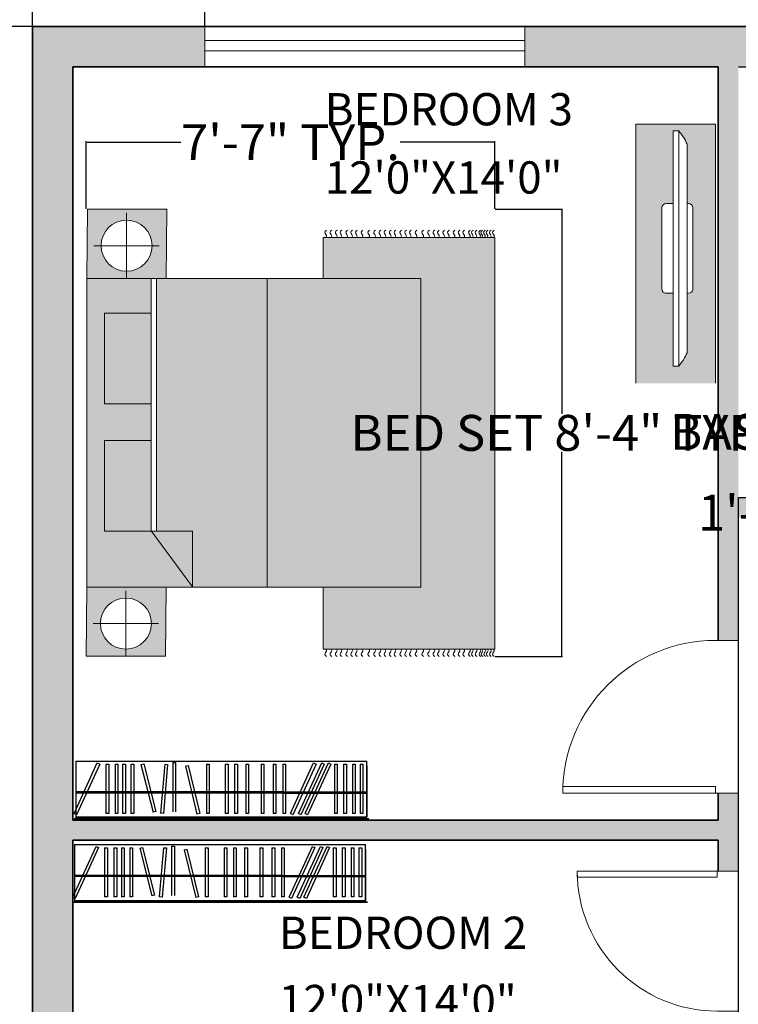
# Model space of a CAD drawing. Units: inches. Extents: x 853 to 1550, y 485 to 1596.
# Tile 13 of 18: x 979 to 1139, y 1208 to 1428. Entities that reach past the tile are written whole.
import ezdxf

# ---------------------------------------------------------------- set-up
doc = ezdxf.new("R2010")
doc.units = ezdxf.units.IN
doc.header["$MEASUREMENT"] = 0
for name, color, linetype, lineweight in [('A-ANNO-DIMS', 2, 'Continuous', 18), ('A-AREA-IDEN', 250, 'Continuous', 18), ('A-DOOR', 4, 'Continuous', 18), ('A-WALL-PATT', 250, 'Continuous', 13), ('closet', 32, 'Continuous', 25), ('furniture', 250, 'Continuous', 18), ('walls', 250, 'Continuous', 35), ('windows', 4, 'Continuous', 18)]:
    doc.layers.add(name, color=color, linetype=linetype, lineweight=lineweight)
doc.layers.add('A-FURN-PATT', color=254, linetype='Continuous', lineweight=13, true_color=0xfeeab9)
doc.styles.get("Standard").update_dxf_attribs({"font": 'arial.ttf'})
doc.dimstyles.get("Standard").update_dxf_attribs({"dimtxt": 8, "dimasz": 0.18, "dimexe": 0.18, "dimexo": 0.0625, "dimgap": 0.09, "dimtad": 0, "dimtih": 1, "dimtoh": 1, "dimzin": 0, "dimdsep": 46, "dimlunit": 3, "dimtxsty": 'Standard', "dimcen": 0.09, "dimadec": 0, "dimazin": 0, "dimtfac": 1, "dimtofl": 0, "dimtmove": 0, "dimatfit": 3, "dimfxl": 1, "dimtolj": 1, "dimtzin": 0, "dimarcsym": 0})

# ---------------------------------------------------------------- blocks, each defined once
blk = doc.blocks.new('CARPET')
at = {"layer": 'furniture'}
for p, q in [((-51.53, -98.11), (-51.53, -55.12)), ((-51.53, -55.12), (-41.27, -55.12)), ((36, -55.12), (51.55, -55.12)), ((51.55, -55.12), (51.55, -98.11)), ((51.55, -98.11), (-51.53, -98.11))]:
    blk.add_line(p, q, dxfattribs=at)
for points, knots in [([(-53.37, -55.99), (-53.22, -55.8), (-52.9, -55.41), (-52.34, -55.8), (-51.89, -56.08), (-51.65, -55.91), (-51.53, -55.83)], [0, 0, 0, 0, 0.653278, 1.290138, 1.740457, 2.114451, 2.114451, 2.114451, 2.114451]), ([(53.37, -55.99), (53.22, -55.8), (52.9, -55.41), (52.34, -55.8), (51.89, -56.08), (51.65, -55.91), (51.53, -55.83)], [0, 0, 0, 0, 0.653278, 1.290138, 1.740457, 2.114451, 2.114451, 2.114451, 2.114451]), ([(-53.37, -57.26), (-53.22, -57.07), (-52.9, -56.67), (-52.34, -57.07), (-51.89, -57.35), (-51.65, -57.17), (-51.53, -57.1)], [0, 0, 0, 0, 0.653278, 1.290138, 1.740457, 2.114451, 2.114451, 2.114451, 2.114451]), ([(-53.37, -58.59), (-53.22, -58.4), (-52.9, -58.01), (-52.34, -58.4), (-51.89, -58.68), (-51.65, -58.5), (-51.53, -58.43)], [0, 0, 0, 0, 0.653278, 1.290138, 1.740457, 2.114451, 2.114451, 2.114451, 2.114451]), ([(53.37, -57.26), (53.22, -57.07), (52.9, -56.67), (52.34, -57.07), (51.89, -57.35), (51.65, -57.17), (51.53, -57.1)], [0, 0, 0, 0, 0.653278, 1.290138, 1.740457, 2.114451, 2.114451, 2.114451, 2.114451]), ([(53.37, -58.59), (53.22, -58.4), (52.9, -58.01), (52.34, -58.4), (51.89, -58.68), (51.65, -58.5), (51.53, -58.43)], [0, 0, 0, 0, 0.653278, 1.290138, 1.740457, 2.114451, 2.114451, 2.114451, 2.114451]), ([(-53.37, -59.78), (-53.22, -59.58), (-52.9, -59.19), (-52.34, -59.58), (-51.89, -59.86), (-51.65, -59.69), (-51.53, -59.61)], [0, 0, 0, 0, 0.653278, 1.290138, 1.740457, 2.114451, 2.114451, 2.114451, 2.114451]), ([(-53.37, -61.22), (-53.22, -61.02), (-52.9, -60.63), (-52.34, -61.02), (-51.89, -61.3), (-51.65, -61.13), (-51.53, -61.05)], [0, 0, 0, 0, 0.653278, 1.290138, 1.740457, 2.114451, 2.114451, 2.114451, 2.114451]), ([(53.37, -59.78), (53.22, -59.58), (52.9, -59.19), (52.34, -59.58), (51.89, -59.86), (51.65, -59.69), (51.53, -59.61)], [0, 0, 0, 0, 0.653278, 1.290138, 1.740457, 2.114451, 2.114451, 2.114451, 2.114451]), ([(53.37, -61.22), (53.22, -61.02), (52.9, -60.63), (52.34, -61.02), (51.89, -61.3), (51.65, -61.13), (51.53, -61.05)], [0, 0, 0, 0, 0.653278, 1.290138, 1.740457, 2.114451, 2.114451, 2.114451, 2.114451]), ([(-53.37, -62.44), (-53.22, -62.25), (-52.9, -61.86), (-52.34, -62.25), (-51.89, -62.53), (-51.65, -62.36), (-51.53, -62.28)], [0, 0, 0, 0, 0.653278, 1.290138, 1.740457, 2.114451, 2.114451, 2.114451, 2.114451]), ([(-53.37, -63.63), (-53.22, -63.43), (-52.9, -63.04), (-52.34, -63.43), (-51.89, -63.72), (-51.65, -63.54), (-51.53, -63.46)], [0, 0, 0, 0, 0.653278, 1.290138, 1.740457, 2.114451, 2.114451, 2.114451, 2.114451]), ([(53.37, -62.44), (53.22, -62.25), (52.9, -61.86), (52.34, -62.25), (51.89, -62.53), (51.65, -62.36), (51.53, -62.28)], [0, 0, 0, 0, 0.653278, 1.290138, 1.740457, 2.114451, 2.114451, 2.114451, 2.114451]), ([(53.37, -63.63), (53.22, -63.43), (52.9, -63.04), (52.34, -63.43), (51.89, -63.72), (51.65, -63.54), (51.53, -63.46)], [0, 0, 0, 0, 0.653278, 1.290138, 1.740457, 2.114451, 2.114451, 2.114451, 2.114451]), ([(-53.37, -65.07), (-53.22, -64.87), (-52.9, -64.48), (-52.34, -64.87), (-51.89, -65.15), (-51.65, -64.98), (-51.53, -64.9)], [0, 0, 0, 0, 0.653278, 1.290138, 1.740457, 2.114451, 2.114451, 2.114451, 2.114451]), ([(-53.37, -66.76), (-53.22, -66.56), (-52.9, -66.17), (-52.34, -66.56), (-51.89, -66.84), (-51.65, -66.67), (-51.53, -66.59)], [0, 0, 0, 0, 0.653278, 1.290138, 1.740457, 2.114451, 2.114451, 2.114451, 2.114451]), ([(53.37, -65.07), (53.22, -64.87), (52.9, -64.48), (52.34, -64.87), (51.89, -65.15), (51.65, -64.98), (51.53, -64.9)], [0, 0, 0, 0, 0.653278, 1.290138, 1.740457, 2.114451, 2.114451, 2.114451, 2.114451]), ([(53.37, -66.76), (53.22, -66.56), (52.9, -66.17), (52.34, -66.56), (51.89, -66.84), (51.65, -66.67), (51.53, -66.59)], [0, 0, 0, 0, 0.653278, 1.290138, 1.740457, 2.114451, 2.114451, 2.114451, 2.114451]), ([(-53.37, -68.2), (-53.22, -68), (-52.9, -67.61), (-52.34, -68), (-51.89, -68.28), (-51.65, -68.11), (-51.53, -68.03)], [0, 0, 0, 0, 0.653278, 1.290138, 1.740457, 2.114451, 2.114451, 2.114451, 2.114451]), ([(53.37, -68.2), (53.22, -68), (52.9, -67.61), (52.34, -68), (51.89, -68.28), (51.65, -68.11), (51.53, -68.03)], [0, 0, 0, 0, 0.653278, 1.290138, 1.740457, 2.114451, 2.114451, 2.114451, 2.114451]), ([(-53.37, -69.53), (-53.22, -69.33), (-52.9, -68.94), (-52.34, -69.33), (-51.89, -69.61), (-51.65, -69.44), (-51.53, -69.36)], [0, 0, 0, 0, 0.653278, 1.290138, 1.740457, 2.114451, 2.114451, 2.114451, 2.114451]), ([(-53.37, -70.79), (-53.22, -70.6), (-52.9, -70.21), (-52.34, -70.6), (-51.89, -70.88), (-51.65, -70.7), (-51.53, -70.63)], [0, 0, 0, 0, 0.653278, 1.290138, 1.740457, 2.114451, 2.114451, 2.114451, 2.114451]), ([(53.37, -69.53), (53.22, -69.33), (52.9, -68.94), (52.34, -69.33), (51.89, -69.61), (51.65, -69.44), (51.53, -69.36)], [0, 0, 0, 0, 0.653278, 1.290138, 1.740457, 2.114451, 2.114451, 2.114451, 2.114451]), ([(53.37, -70.79), (53.22, -70.6), (52.9, -70.21), (52.34, -70.6), (51.89, -70.88), (51.65, -70.7), (51.53, -70.63)], [0, 0, 0, 0, 0.653278, 1.290138, 1.740457, 2.114451, 2.114451, 2.114451, 2.114451]), ([(-53.37, -72.12), (-53.22, -71.93), (-52.9, -71.54), (-52.34, -71.93), (-51.89, -72.21), (-51.65, -72.04), (-51.53, -71.96)], [0, 0, 0, 0, 0.653278, 1.290138, 1.740457, 2.114451, 2.114451, 2.114451, 2.114451]), ([(-53.37, -73.31), (-53.22, -73.11), (-52.9, -72.72), (-52.34, -73.11), (-51.89, -73.4), (-51.65, -73.22), (-51.53, -73.14)], [0, 0, 0, 0, 0.653278, 1.290138, 1.740457, 2.114451, 2.114451, 2.114451, 2.114451]), ([(53.37, -72.12), (53.22, -71.93), (52.9, -71.54), (52.34, -71.93), (51.89, -72.21), (51.65, -72.04), (51.53, -71.96)], [0, 0, 0, 0, 0.653278, 1.290138, 1.740457, 2.114451, 2.114451, 2.114451, 2.114451]), ([(53.37, -73.31), (53.22, -73.11), (52.9, -72.72), (52.34, -73.11), (51.89, -73.4), (51.65, -73.22), (51.53, -73.14)], [0, 0, 0, 0, 0.653278, 1.290138, 1.740457, 2.114451, 2.114451, 2.114451, 2.114451]), ([(-53.37, -74.75), (-53.22, -74.55), (-52.9, -74.16), (-52.34, -74.55), (-51.89, -74.83), (-51.65, -74.66), (-51.53, -74.58)], [0, 0, 0, 0, 0.653278, 1.290138, 1.740457, 2.114451, 2.114451, 2.114451, 2.114451]), ([(-53.37, -75.98), (-53.22, -75.78), (-52.9, -75.39), (-52.34, -75.78), (-51.89, -76.06), (-51.65, -75.89), (-51.53, -75.81)], [0, 0, 0, 0, 0.653278, 1.290138, 1.740457, 2.114451, 2.114451, 2.114451, 2.114451]), ([(53.37, -74.75), (53.22, -74.55), (52.9, -74.16), (52.34, -74.55), (51.89, -74.83), (51.65, -74.66), (51.53, -74.58)], [0, 0, 0, 0, 0.653278, 1.290138, 1.740457, 2.114451, 2.114451, 2.114451, 2.114451]), ([(53.37, -75.98), (53.22, -75.78), (52.9, -75.39), (52.34, -75.78), (51.89, -76.06), (51.65, -75.89), (51.53, -75.81)], [0, 0, 0, 0, 0.653278, 1.290138, 1.740457, 2.114451, 2.114451, 2.114451, 2.114451]), ([(-53.37, -77.16), (-53.22, -76.96), (-52.9, -76.57), (-52.34, -76.96), (-51.89, -77.25), (-51.65, -77.07), (-51.53, -76.99)], [0, 0, 0, 0, 0.653278, 1.290138, 1.740457, 2.114451, 2.114451, 2.114451, 2.114451]), ([(-53.37, -78.6), (-53.22, -78.4), (-52.9, -78.01), (-52.34, -78.4), (-51.89, -78.68), (-51.65, -78.51), (-51.53, -78.43)], [0, 0, 0, 0, 0.653278, 1.290138, 1.740457, 2.114451, 2.114451, 2.114451, 2.114451]), ([(53.37, -77.16), (53.22, -76.96), (52.9, -76.57), (52.34, -76.96), (51.89, -77.25), (51.65, -77.07), (51.53, -76.99)], [0, 0, 0, 0, 0.653278, 1.290138, 1.740457, 2.114451, 2.114451, 2.114451, 2.114451]), ([(53.37, -78.6), (53.22, -78.4), (52.9, -78.01), (52.34, -78.4), (51.89, -78.68), (51.65, -78.51), (51.53, -78.43)], [0, 0, 0, 0, 0.653278, 1.290138, 1.740457, 2.114451, 2.114451, 2.114451, 2.114451]), ([(-53.37, -80.29), (-53.22, -80.09), (-52.9, -79.7), (-52.34, -80.09), (-51.89, -80.37), (-51.65, -80.2), (-51.53, -80.12)], [0, 0, 0, 0, 0.653278, 1.290138, 1.740457, 2.114451, 2.114451, 2.114451, 2.114451]), ([(-53.37, -81.73), (-53.22, -81.53), (-52.9, -81.14), (-52.34, -81.53), (-51.89, -81.81), (-51.65, -81.64), (-51.53, -81.56)], [0, 0, 0, 0, 0.653278, 1.290138, 1.740457, 2.114451, 2.114451, 2.114451, 2.114451]), ([(53.37, -80.29), (53.22, -80.09), (52.9, -79.7), (52.34, -80.09), (51.89, -80.37), (51.65, -80.2), (51.53, -80.12)], [0, 0, 0, 0, 0.653278, 1.290138, 1.740457, 2.114451, 2.114451, 2.114451, 2.114451]), ([(53.37, -81.73), (53.22, -81.53), (52.9, -81.14), (52.34, -81.53), (51.89, -81.81), (51.65, -81.64), (51.53, -81.56)], [0, 0, 0, 0, 0.653278, 1.290138, 1.740457, 2.114451, 2.114451, 2.114451, 2.114451]), ([(-53.37, -83.06), (-53.22, -82.86), (-52.9, -82.47), (-52.34, -82.86), (-51.89, -83.14), (-51.65, -82.97), (-51.53, -82.89)], [0, 0, 0, 0, 0.653278, 1.290138, 1.740457, 2.114451, 2.114451, 2.114451, 2.114451]), ([(-53.37, -84.18), (-53.22, -83.99), (-52.9, -83.6), (-52.34, -83.99), (-51.89, -84.27), (-51.65, -84.09), (-51.53, -84.02)], [0, 0, 0, 0, 0.653278, 1.290138, 1.740457, 2.114451, 2.114451, 2.114451, 2.114451]), ([(53.37, -83.06), (53.22, -82.86), (52.9, -82.47), (52.34, -82.86), (51.89, -83.14), (51.65, -82.97), (51.53, -82.89)], [0, 0, 0, 0, 0.653278, 1.290138, 1.740457, 2.114451, 2.114451, 2.114451, 2.114451]), ([(53.37, -84.18), (53.22, -83.99), (52.9, -83.6), (52.34, -83.99), (51.89, -84.27), (51.65, -84.09), (51.53, -84.02)], [0, 0, 0, 0, 0.653278, 1.290138, 1.740457, 2.114451, 2.114451, 2.114451, 2.114451]), ([(-53.37, -85.51), (-53.22, -85.32), (-52.9, -84.93), (-52.34, -85.32), (-51.89, -85.6), (-51.65, -85.42), (-51.53, -85.35)], [0, 0, 0, 0, 0.653278, 1.290138, 1.740457, 2.114451, 2.114451, 2.114451, 2.114451]), ([(-53.37, -86.7), (-53.22, -86.5), (-52.9, -86.11), (-52.34, -86.5), (-51.89, -86.78), (-51.65, -86.61), (-51.53, -86.53)], [0, 0, 0, 0, 0.653278, 1.290138, 1.740457, 2.114451, 2.114451, 2.114451, 2.114451]), ([(53.37, -85.51), (53.22, -85.32), (52.9, -84.93), (52.34, -85.32), (51.89, -85.6), (51.65, -85.42), (51.53, -85.35)], [0, 0, 0, 0, 0.653278, 1.290138, 1.740457, 2.114451, 2.114451, 2.114451, 2.114451]), ([(53.37, -86.7), (53.22, -86.5), (52.9, -86.11), (52.34, -86.5), (51.89, -86.78), (51.65, -86.61), (51.53, -86.53)], [0, 0, 0, 0, 0.653278, 1.290138, 1.740457, 2.114451, 2.114451, 2.114451, 2.114451]), ([(-53.37, -88.14), (-53.22, -87.94), (-52.9, -87.55), (-52.34, -87.94), (-51.89, -88.22), (-51.65, -88.05), (-51.53, -87.97)], [0, 0, 0, 0, 0.653278, 1.290138, 1.740457, 2.114451, 2.114451, 2.114451, 2.114451]), ([(53.37, -88.14), (53.22, -87.94), (52.9, -87.55), (52.34, -87.94), (51.89, -88.22), (51.65, -88.05), (51.53, -87.97)], [0, 0, 0, 0, 0.653278, 1.290138, 1.740457, 2.114451, 2.114451, 2.114451, 2.114451]), ([(-53.37, -89.36), (-53.22, -89.17), (-52.9, -88.78), (-52.34, -89.17), (-51.89, -89.45), (-51.65, -89.28), (-51.53, -89.2)], [0, 0, 0, 0, 0.653278, 1.290138, 1.740457, 2.114451, 2.114451, 2.114451, 2.114451]), ([(-53.37, -90.55), (-53.22, -90.35), (-52.9, -89.96), (-52.34, -90.35), (-51.89, -90.64), (-51.65, -90.46), (-51.53, -90.38)], [0, 0, 0, 0, 0.653278, 1.290138, 1.740457, 2.114451, 2.114451, 2.114451, 2.114451]), ([(53.37, -89.36), (53.22, -89.17), (52.9, -88.78), (52.34, -89.17), (51.89, -89.45), (51.65, -89.28), (51.53, -89.2)], [0, 0, 0, 0, 0.653278, 1.290138, 1.740457, 2.114451, 2.114451, 2.114451, 2.114451]), ([(53.37, -90.55), (53.22, -90.35), (52.9, -89.96), (52.34, -90.35), (51.9, -90.63), (51.66, -90.47), (51.55, -90.4)], [0, 0, 0, 0, 0.653278, 1.290138, 1.740457, 2.0926, 2.0926, 2.0926, 2.0926]), ([(-53.37, -91.99), (-53.22, -91.79), (-52.9, -91.4), (-52.34, -91.79), (-51.89, -92.07), (-51.65, -91.9), (-51.53, -91.82)], [0, 0, 0, 0, 0.653278, 1.290138, 1.740457, 2.114451, 2.114451, 2.114451, 2.114451]), ([(-53.37, -92.69), (-53.22, -92.48), (-52.9, -92.08), (-52.35, -92.49), (-51.89, -92.77), (-51.65, -92.6), (-51.53, -92.52)], [0, 0, 0, 0, 0.663904, 1.307406, 1.757725, 2.131719, 2.131719, 2.131719, 2.131719]), ([(-53.37, -93.61), (-53.22, -93.42), (-52.9, -93.03), (-52.34, -93.42), (-51.89, -93.7), (-51.65, -93.52), (-51.53, -93.45)], [0, 0, 0, 0, 0.653278, 1.290138, 1.740457, 2.114451, 2.114451, 2.114451, 2.114451]), ([(53.37, -91.99), (53.22, -91.79), (52.9, -91.4), (52.34, -91.79), (51.9, -92.07), (51.66, -91.91), (51.55, -91.83)], [0, 0, 0, 0, 0.653278, 1.290138, 1.740457, 2.0926, 2.0926, 2.0926, 2.0926]), ([(53.37, -92.69), (53.22, -92.49), (52.9, -92.09), (52.34, -92.49), (51.9, -92.77), (51.66, -92.61), (51.55, -92.53)], [0, 0, 0, 0, 0.656792, 1.295826, 1.746145, 2.098292, 2.098292, 2.098292, 2.098292]), ([(53.37, -93.66), (53.22, -93.46), (52.9, -93.07), (52.34, -93.46), (51.9, -93.74), (51.66, -93.58), (51.55, -93.5)], [0, 0, 0, 0, 0.653278, 1.290138, 1.740457, 2.0926, 2.0926, 2.0926, 2.0926]), ([(-53.37, -94.55), (-53.22, -94.35), (-52.9, -93.96), (-52.34, -94.35), (-51.89, -94.63), (-51.65, -94.46), (-51.53, -94.38)], [0, 0, 0, 0, 0.653278, 1.290138, 1.740457, 2.114451, 2.114451, 2.114451, 2.114451]), ([(-53.37, -95.05), (-53.22, -94.85), (-52.9, -94.46), (-52.34, -94.85), (-51.89, -95.14), (-51.65, -94.96), (-51.53, -94.88)], [0, 0, 0, 0, 0.653278, 1.290138, 1.740457, 2.114451, 2.114451, 2.114451, 2.114451]), ([(-53.37, -95.73), (-53.22, -95.54), (-52.9, -95.15), (-52.34, -95.54), (-51.89, -95.82), (-51.65, -95.65), (-51.53, -95.57)], [0, 0, 0, 0, 0.653278, 1.290138, 1.740457, 2.114451, 2.114451, 2.114451, 2.114451]), ([(-53.37, -96.38), (-53.22, -96.18), (-52.9, -95.79), (-52.34, -96.18), (-51.89, -96.47), (-51.65, -96.29), (-51.53, -96.21)], [0, 0, 0, 0, 0.653278, 1.290138, 1.740457, 2.114451, 2.114451, 2.114451, 2.114451]), ([(53.37, -95.78), (53.22, -95.58), (52.9, -95.19), (52.34, -95.58), (51.89, -95.86), (51.65, -95.69), (51.53, -95.61)], [0, 0, 0, 0, 0.653278, 1.290138, 1.740457, 2.114451, 2.114451, 2.114451, 2.114451]), ([(53.37, -96.43), (53.22, -96.23), (52.9, -95.84), (52.34, -96.23), (51.89, -96.51), (51.65, -96.34), (51.53, -96.26)], [0, 0, 0, 0, 0.653278, 1.290138, 1.740457, 2.114451, 2.114451, 2.114451, 2.114451]), ([(53.37, -94.59), (53.22, -94.4), (52.9, -94.01), (52.34, -94.4), (51.9, -94.68), (51.66, -94.51), (51.55, -94.44)], [0, 0, 0, 0, 0.653278, 1.290138, 1.740457, 2.0926, 2.0926, 2.0926, 2.0926]), ([(53.37, -95.1), (53.22, -94.9), (52.9, -94.51), (52.34, -94.9), (51.9, -95.18), (51.66, -95.02), (51.55, -94.94)], [0, 0, 0, 0, 0.653278, 1.290138, 1.740457, 2.0926, 2.0926, 2.0926, 2.0926]), ([(-53.37, -97.17), (-53.22, -96.98), (-52.9, -96.59), (-52.34, -96.98), (-51.89, -97.26), (-51.65, -97.08), (-51.53, -97.01)], [0, 0, 0, 0, 0.653278, 1.290138, 1.740457, 2.114451, 2.114451, 2.114451, 2.114451]), ([(-53.37, -97.99), (-53.22, -97.79), (-52.9, -97.4), (-52.34, -97.79), (-51.89, -98.08), (-51.65, -97.9), (-51.53, -97.82)], [0, 0, 0, 0, 0.653278, 1.290138, 1.740457, 2.114451, 2.114451, 2.114451, 2.114451]), ([(53.37, -97.22), (53.22, -97.02), (52.9, -96.63), (52.34, -97.02), (51.89, -97.3), (51.65, -97.13), (51.53, -97.05)], [0, 0, 0, 0, 0.653278, 1.290138, 1.740457, 2.114451, 2.114451, 2.114451, 2.114451]), ([(53.37, -97.99), (53.22, -97.79), (52.9, -97.4), (52.34, -97.79), (51.89, -98.08), (51.65, -97.9), (51.53, -97.82)], [0, 0, 0, 0, 0.653278, 1.290138, 1.740457, 2.114451, 2.114451, 2.114451, 2.114451])]:
    blk.add_open_spline(points, degree=3, knots=knots, dxfattribs=at)
blk = doc.blocks.new('A$C58D270C6')
at = {"layer": 'furniture'}
for p, q in [((9.09, 124.13), (9.09, 108.87)), ((1.46, 116.5), (16.73, 116.5)), ((42.08, 108), (42.08, 36)), ((14.97, 94.84), (24.62, 107.92)), ((24.62, 94.93), (24.62, 107.92)), ((14.97, 94.93), (24.62, 94.93)), ((14.97, 94.84), (14.97, 36)), ((16.22, 94.93), (16.22, 36)), ((9.25, 36), (9.25, 20.74)), ((1.62, 28.37), (16.88, 28.37))]:
    blk.add_line(p, q, dxfattribs=at)
for points in [[(18.5, 108), (18.34, 124.13), (-0.16, 124.13), (0, 108)], [(0, 108), (77.91, 108), (77.91, 36), (0, 36)], [(4.09, 94.93), (14.97, 94.93), (14.97, 73.83), (4.09, 73.83)], [(4.09, 65.23), (14.97, 65.23), (14.97, 44.13), (4.09, 44.13)], [(18.65, 19.87), (18.5, 36), (0, 36), (0.16, 19.87)]]:
    blk.add_lwpolyline(points, close=True, dxfattribs=at)
for centre in [(9.09, 116.5), (9.25, 28.37)]:
    blk.add_circle(centre, 5.95, dxfattribs=at)
at = {"layer": 'furniture', "xscale": 0.9312884925094044, "yscale": 0.9312884925094044, "zscale": 0.9312884925094044, "rotation": 90}
blk.add_blockref('CARPET', (3.79, 74.47), dxfattribs=at)
blk = doc.blocks.new('*U10')
for p, q in [((0, 0), (0, -6)), ((40, 0), (40, -6))]:
    blk.add_line(p, q)
blk.add_lwpolyline([(0, 0), (0, 40), (1.75, 40), (1.75, 0)], close=True)
blk.add_arc((0, 0), 40, 0, 90)
blk = doc.blocks.new('WIN-71IN')
for p, q in [((0, 9), (0, 0)), ((71.43, 9), (0, 9)), ((0, 9), (0, 5.92)), ((71.43, 0), (71.43, 9)), ((0, 5.92), (71.43, 5.92)), ((71.43, 5.92), (71.43, 3.59)), ((71.43, 3.59), (0, 3.59)), ((0, 0), (71.43, 0))]:
    blk.add_line(p, q)
blk = doc.blocks.new('closet')
at = {"layer": 'closet'}
for p, q in [((-0.71, -5.58), (5.59, 8.19)), ((5.59, 8.19), (6.27, 7.88)), ((26.09, 8.25), (26.09, -5.1)), ((26.84, 8.25), (26.84, -5.1)), ((57.99, -5.58), (64.3, 8.19)), ((60.19, -5.58), (66.49, 8.19)), ((62, -5.58), (68.3, 8.19)), ((-0.23, 7.39), (-0.23, -6.57)), ((6.27, 7.88), (-0.04, -5.89)), ((7.92, 7.84), (8.68, 7.84)), ((7.92, 7.84), (7.92, -5.51)), ((8.68, 7.84), (8.68, -5.51)), ((10.44, 7.84), (11.2, 7.84)), ((10.44, 7.84), (10.44, -5.51)), ((11.2, 7.84), (11.2, -5.51)), ((12.45, 7.84), (13.21, 7.84)), ((12.45, 7.84), (12.45, -5.51)), ((13.21, 7.84), (13.21, -5.51)), ((14.71, 7.84), (15.47, 7.84)), ((14.71, 7.84), (14.71, -5.51)), ((15.47, 7.84), (15.47, -5.51)), ((17.44, 7.75), (18.17, 7.93)), ((17.44, 7.75), (20.73, -5.2)), ((18.17, 7.93), (21.46, -5.01)), ((23.92, 7.84), (22.75, -5.46)), ((24.67, 7.78), (23.51, -5.53)), ((23.92, 7.84), (24.67, 7.78)), ((29.49, 7.29), (32.64, -5.69)), ((30.22, 7.46), (33.37, -5.51)), ((35.23, 7.84), (35.23, -5.51)), ((35.99, 7.84), (35.99, -5.51)), ((40.33, 7.84), (40.33, -5.51)), ((41.08, 7.84), (41.08, -5.51)), ((42.85, 7.84), (42.85, -5.51)), ((43.61, 7.84), (43.61, -5.51)), ((45.9, 7.84), (45.9, -5.51)), ((46.65, 7.84), (46.65, -5.51)), ((50.07, 7.84), (50.07, -5.51)), ((50.82, 7.84), (50.82, -5.51)), ((53.32, 7.84), (53.32, -5.51)), ((54.08, 7.84), (54.08, -5.51)), ((55.9, 7.84), (55.9, -5.51)), ((56.65, 7.84), (56.65, -5.51)), ((64.97, 7.88), (58.67, -5.89)), ((67.17, 7.88), (60.87, -5.89)), ((68.98, 7.88), (62.67, -5.89)), ((69.96, 7.84), (69.96, -5.51)), ((70.72, 7.84), (70.72, -5.51)), ((72.43, 7.84), (72.43, -5.51)), ((73.19, 7.84), (73.19, -5.51)), ((74.82, 7.84), (74.82, -5.51)), ((75.57, 7.84), (75.57, -5.51)), ((76.94, 7.84), (76.94, -5.51)), ((77.69, 7.84), (77.69, -5.51)), ((56.23, 0.33), (0, 0.33)), ((56.2, 0), (0, 0)), ((56.2, 0), (78.76, 0)), ((56.23, 0.33), (78.76, 0.33)), ((21.46, -5.01), (20.73, -5.2)), ((-0.04, -5.89), (-0.71, -5.58)), ((23.51, -5.53), (22.75, -5.46)), ((33.37, -5.51), (32.64, -5.69)), ((35.99, -5.51), (35.23, -5.51)), ((41.08, -5.51), (40.33, -5.51)), ((43.61, -5.51), (42.85, -5.51)), ((46.65, -5.51), (45.9, -5.51)), ((50.82, -5.51), (50.07, -5.51)), ((54.08, -5.51), (53.32, -5.51)), ((56.65, -5.51), (55.9, -5.51)), ((58.67, -5.89), (57.99, -5.58)), ((60.87, -5.89), (60.19, -5.58)), ((62.67, -5.89), (62, -5.58)), ((70.72, -5.51), (69.96, -5.51)), ((73.19, -5.51), (72.43, -5.51)), ((75.57, -5.51), (74.82, -5.51)), ((77.69, -5.51), (76.94, -5.51))]:
    blk.add_line(p, q, dxfattribs=at)
blk = doc.blocks.new('rotated closet')
at = {"layer": 'closet'}
for p, q in [((26.32, 0.86), (27.07, 0.86)), ((29.72, -0.11), (30.45, 0.07)), ((35.46, 0.45), (36.22, 0.45)), ((40.56, 0.45), (41.31, 0.45)), ((43.08, 0.45), (43.84, 0.45)), ((46.13, 0.45), (46.88, 0.45)), ((50.3, 0.45), (51.05, 0.45)), ((53.56, 0.45), (54.31, 0.45)), ((56.13, 0.45), (56.88, 0.45)), ((64.53, 0.8), (65.2, 0.49)), ((66.72, 0.8), (67.4, 0.49)), ((68.53, 0.8), (69.21, 0.49)), ((70.19, 0.45), (70.95, 0.45)), ((72.66, 0.45), (73.42, 0.45)), ((75.05, 0.45), (75.81, 0.45)), ((77.17, 0.45), (77.92, 0.45)), ((78.99, 0), (78.99, -13.96)), ((8.91, -12.91), (8.15, -12.91)), ((11.43, -12.91), (10.67, -12.91)), ((13.44, -12.91), (12.68, -12.91)), ((15.7, -12.91), (14.94, -12.91)), ((-0.46, -14.27), (79.54, -14.27)), ((0, -13.96), (78.99, -13.96))]:
    blk.add_line(p, q, dxfattribs=at)
blk.add_blockref('closet', (0.23, -7.39), dxfattribs=at)
blk = doc.blocks.new('WARDROBE-FRAMED')
for p, q in [((0.4, 12.8), (65.33, 12.8)), ((0.4, 12.8), (0.4, 0.26)), ((65.33, 0.26), (65.33, 12.8)), ((0.02, 0), (65.79, 0)), ((65.33, 0.26), (0.4, 0.26)), ((0.4, 0.26), (0.4, 0))]:
    blk.add_line(p, q)
at = {"xscale": 0.8221057635095903, "yscale": 0.8221057635095903, "zscale": 0.8221057635095903, "rotation": 359.9999999992008}
blk.add_blockref('rotated closet', (0.4, 11.74), dxfattribs=at)
blk = doc.blocks.new('PLASMA-LARGE')
at = {"layer": 'furniture'}
for p, q in [((-7.26, 0), (7.26, 0)), ((-18.61, -1), (18.61, -1)), ((-8, -1), (-8, -0.74)), ((8, -1), (8, -0.74)), ((-21, -2.5), (21, -2.5)), ((-21, -2.5), (-21, -3.5)), ((-21, -3.5), (21, -3.5)), ((-8, -3.5), (-8, -4.76)), ((8, -3.5), (8, -4.76)), ((21, -2.5), (21, -3.5)), ((-7.26, -5.5), (7.26, -5.5))]:
    blk.add_line(p, q, dxfattribs=at)
for centre, radius, start, end in [((-7.26, -0.74), 0.744, 90, 180), ((7.26, -0.74), 0.744, 0, 90), ((-13.97, -11.05), 11.07, 114.7602, 129.4175), ((13.97, -11.05), 11.07, 50.5825, 65.2398), ((-7.26, -4.76), 0.744, 180, 270), ((7.26, -4.76), 0.744, 270, 0)]:
    blk.add_arc(centre, radius, start, end, dxfattribs=at)
blk = doc.blocks.new('TV-CONSOLE')
for p, q in [((0, 0), (0, 57.83)), ((0, 57.83), (17.81, 57.83)), ((17.81, 57.83), (17.81, 0))]:
    blk.add_line(p, q)
at = {"xscale": 1.249763490704796, "yscale": 1.249763490704796, "zscale": 1.249763490704796, "rotation": 270}
blk.add_blockref('PLASMA-LARGE', (12.71, 30.08), dxfattribs=at)
blk = doc.blocks.new('*D37')
at = {"layer": 'A-ANNO-DIMS', "color": 0, "lineweight": -2, "transparency": 16777216}
for p, q in [((1085.15, 1385.39), (1100.23, 1385.39)), ((1100.05, 1385.21), (1100.05, 1339.74)), ((1100.05, 1285.81), (1100.05, 1331.29)), ((1085.15, 1285.63), (1100.23, 1285.63))]:
    blk.add_line(p, q, dxfattribs=at)
at = {"layer": 'A-ANNO-DIMS', "color": 0, "transparency": 16777216}
for points in [[(1100.02, 1385.21), (1100.08, 1385.21), (1100.05, 1385.39)], [(1100.02, 1285.81), (1100.08, 1285.81), (1100.05, 1285.63)]]:
    blk.add_solid(points, dxfattribs=at)
at = {"layer": 'Defpoints', "color": 0, "transparency": 16777216}
for p in [(1085.09, 1385.39), (1085.09, 1285.63), (1100.05, 1285.63)]:
    blk.add_point(p, dxfattribs=at)
at = {"layer": 'A-ANNO-DIMS', "color": 0, "transparency": 16777216, "insert": (1100.05, 1335.51), "char_height": 8, "attachment_point": 5}
blk.add_mtext('\\A1;BED SET 8\'-4" TYP.', dxfattribs=at)
blk = doc.blocks.new('*D38')
at = {"layer": 'A-ANNO-DIMS', "color": 0, "lineweight": -2, "transparency": 16777216}
for p, q in [((993.93, 1385.46), (993.93, 1400.54)), ((994.11, 1400.36), (1015.07, 1400.36)), ((1084.91, 1400.36), (1063.95, 1400.36)), ((1085.09, 1385.46), (1085.09, 1400.54))]:
    blk.add_line(p, q, dxfattribs=at)
at = {"layer": 'A-ANNO-DIMS', "color": 0, "transparency": 16777216}
for points in [[(994.11, 1400.39), (994.11, 1400.33), (993.93, 1400.36)], [(1084.91, 1400.39), (1084.91, 1400.33), (1085.09, 1400.36)]]:
    blk.add_solid(points, dxfattribs=at)
at = {"layer": 'Defpoints', "color": 0, "transparency": 16777216}
for p in [(1085.09, 1400.36), (993.93, 1385.39), (1085.09, 1385.39)]:
    blk.add_point(p, dxfattribs=at)
at = {"layer": 'A-ANNO-DIMS', "color": 0, "transparency": 16777216, "insert": (1039.51, 1400.36), "char_height": 8, "attachment_point": 5}
blk.add_mtext('\\A1;7\'-7" TYP.', dxfattribs=at)
blk = doc.blocks.new('*D39')
at = {"layer": 'A-ANNO-DIMS', "color": 0, "lineweight": -2, "transparency": 16777216}
for p, q in [((1179.06, 1349.58), (1174.79, 1349.58)), ((1174.97, 1349.4), (1174.97, 1339.96)), ((1174.97, 1322.06), (1174.97, 1331.5)), ((1179.06, 1321.88), (1174.79, 1321.88))]:
    blk.add_line(p, q, dxfattribs=at)
at = {"layer": 'A-ANNO-DIMS', "color": 0, "transparency": 16777216}
for points in [[(1174.94, 1349.4), (1175, 1349.4), (1174.97, 1349.58)], [(1174.94, 1322.06), (1175, 1322.06), (1174.97, 1321.88)]]:
    blk.add_solid(points, dxfattribs=at)
at = {"layer": 'Defpoints', "color": 0, "transparency": 16777216}
for p in [(1174.97, 1349.58), (1179.12, 1349.58), (1179.12, 1321.88)]:
    blk.add_point(p, dxfattribs=at)
at = {"layer": 'A-ANNO-DIMS', "color": 0, "transparency": 16777216, "insert": (1174.97, 1335.73), "char_height": 8, "attachment_point": 5}
blk.add_mtext('\\A1;BASIN 2\'-3 1/2" TYP.', dxfattribs=at)
blk = doc.blocks.new('*D40')
at = {"layer": 'A-ANNO-DIMS', "color": 0, "lineweight": -2, "transparency": 16777216}
for p, q in [((1179.12, 1321.82), (1179.12, 1317.54)), ((1198.3, 1321.82), (1198.3, 1317.54)), ((1179.12, 1317.72), (1178.94, 1317.72)), ((1198.12, 1317.72), (1179.3, 1317.72))]:
    blk.add_line(p, q, dxfattribs=at)
at = {"layer": 'A-ANNO-DIMS', "color": 0, "transparency": 16777216}
for points in [[(1179.3, 1317.75), (1179.3, 1317.69), (1179.12, 1317.72)], [(1198.12, 1317.75), (1198.12, 1317.69), (1198.3, 1317.72)]]:
    blk.add_solid(points, dxfattribs=at)
at = {"layer": 'Defpoints', "color": 0, "transparency": 16777216}
for p in [(1179.12, 1321.88), (1198.3, 1321.88), (1179.12, 1317.72)]:
    blk.add_point(p, dxfattribs=at)
at = {"layer": 'A-ANNO-DIMS', "color": 0, "transparency": 16777216, "insert": (1154.85, 1317.72), "char_height": 8, "attachment_point": 5}
blk.add_mtext('\\A1;1\'-7" TYP.', dxfattribs=at)
blk = doc.blocks.new('*D69')
at = {"layer": 'A-ANNO-DIMS', "color": 0, "lineweight": -2, "transparency": 16777216}
for p, q in [((981.94, 1426.19), (981.94, 1584.65)), ((982.12, 1584.47), (1184.11, 1584.47)), ((1413.76, 1584.47), (1211.77, 1584.47)), ((1413.94, 1426.19), (1413.94, 1584.65))]:
    blk.add_line(p, q, dxfattribs=at)
at = {"layer": 'A-ANNO-DIMS', "color": 0, "transparency": 16777216}
for points in [[(982.12, 1584.5), (982.12, 1584.44), (981.94, 1584.47)], [(1413.76, 1584.5), (1413.76, 1584.44), (1413.94, 1584.47)]]:
    blk.add_solid(points, dxfattribs=at)
at = {"layer": 'Defpoints', "color": 0, "transparency": 16777216}
for p in [(1413.94, 1584.47), (981.94, 1426.13), (1413.94, 1426.13)]:
    blk.add_point(p, dxfattribs=at)
at = {"layer": 'A-ANNO-DIMS', "color": 0, "transparency": 16777216, "insert": (1197.94, 1584.47), "char_height": 8, "attachment_point": 5}
blk.add_mtext('\\A1;36\'-0"', dxfattribs=at)
blk = doc.blocks.new('*D70')
at = {"layer": 'A-ANNO-DIMS', "color": 0, "lineweight": -2, "transparency": 16777216}
for p, q in [((981.87, 1426.13), (877.09, 1426.13)), ((877.27, 1425.95), (877.27, 1067.22)), ((877.27, 700.05), (877.27, 1058.77)), ((1110.88, 699.87), (877.09, 699.87))]:
    blk.add_line(p, q, dxfattribs=at)
at = {"layer": 'A-ANNO-DIMS', "color": 0, "transparency": 16777216}
for points in [[(877.24, 1425.95), (877.3, 1425.95), (877.27, 1426.13)], [(877.24, 700.05), (877.3, 700.05), (877.27, 699.87)]]:
    blk.add_solid(points, dxfattribs=at)
at = {"layer": 'Defpoints', "color": 0, "transparency": 16777216}
for p in [(981.94, 1426.13), (877.27, 699.87), (1110.94, 699.87)]:
    blk.add_point(p, dxfattribs=at)
at = {"layer": 'A-ANNO-DIMS', "color": 0, "transparency": 16777216, "insert": (877.27, 1063), "char_height": 8, "attachment_point": 5}
blk.add_mtext('\\A1;60\'-6 1/2"', dxfattribs=at)
blk = doc.blocks.new('*D72')
at = {"layer": 'A-ANNO-DIMS', "color": 0, "lineweight": -2, "transparency": 16777216}
for p, q in [((1139.44, 1321.07), (1139.44, 497.1)), ((1199.44, 1321.07), (1199.44, 497.1)), ((1139.62, 497.28), (1158.71, 497.28)), ((1199.26, 497.28), (1180.16, 497.28))]:
    blk.add_line(p, q, dxfattribs=at)
at = {"layer": 'A-ANNO-DIMS', "color": 0, "transparency": 16777216}
for points in [[(1139.62, 497.31), (1139.62, 497.25), (1139.44, 497.28)], [(1199.26, 497.31), (1199.26, 497.25), (1199.44, 497.28)]]:
    blk.add_solid(points, dxfattribs=at)
at = {"layer": 'Defpoints', "color": 0, "transparency": 16777216}
for p in [(1139.44, 1321.13), (1199.44, 1321.13), (1199.44, 497.28)]:
    blk.add_point(p, dxfattribs=at)
at = {"layer": 'A-ANNO-DIMS', "color": 0, "transparency": 16777216, "insert": (1169.44, 497.28), "char_height": 8, "attachment_point": 5}
blk.add_mtext('\\A1;5\'-0"', dxfattribs=at)
blk = doc.blocks.new('*D73')
at = {"layer": 'A-ANNO-DIMS', "color": 0, "lineweight": -2, "transparency": 16777216}
for p, q in [((1139.5, 1417.13), (1526.24, 1417.13)), ((1526.06, 1416.95), (1526.06, 1373.3)), ((1526.06, 1321.31), (1526.06, 1364.95)), ((1139.5, 1321.13), (1526.24, 1321.13))]:
    blk.add_line(p, q, dxfattribs=at)
at = {"layer": 'A-ANNO-DIMS', "color": 0, "transparency": 16777216}
for points in [[(1526.03, 1416.95), (1526.09, 1416.95), (1526.06, 1417.13)], [(1526.03, 1321.31), (1526.09, 1321.31), (1526.06, 1321.13)]]:
    blk.add_solid(points, dxfattribs=at)
at = {"layer": 'Defpoints', "color": 0, "transparency": 16777216}
for p in [(1139.44, 1417.13), (1139.44, 1321.13), (1526.06, 1321.13)]:
    blk.add_point(p, dxfattribs=at)
at = {"layer": 'A-ANNO-DIMS', "color": 0, "transparency": 16777216, "insert": (1526.06, 1369.13), "char_height": 8, "attachment_point": 5}
blk.add_mtext('\\A1;8\'-0"', dxfattribs=at)
blk = doc.blocks.new('*D82')
at = {"layer": 'A-ANNO-DIMS', "color": 0, "lineweight": -2, "transparency": 16777216}
for p, q in [((981.94, 1426.19), (981.94, 1584.65)), ((982.12, 1584.47), (1020.22, 1584.47)), ((1020.4, 1426.19), (1020.4, 1584.65)), ((1020.4, 1584.47), (1020.58, 1584.47))]:
    blk.add_line(p, q, dxfattribs=at)
at = {"layer": 'A-ANNO-DIMS', "color": 0, "transparency": 16777216}
for points in [[(982.12, 1584.5), (982.12, 1584.44), (981.94, 1584.47)], [(1020.22, 1584.5), (1020.22, 1584.44), (1020.4, 1584.47)]]:
    blk.add_solid(points, dxfattribs=at)
at = {"layer": 'Defpoints', "color": 0, "transparency": 16777216}
for p in [(1020.4, 1584.47), (981.94, 1426.13), (1020.4, 1426.13)]:
    blk.add_point(p, dxfattribs=at)
at = {"layer": 'A-ANNO-DIMS', "color": 0, "transparency": 16777216, "insert": (1040.62, 1584.47), "char_height": 8, "attachment_point": 5}
blk.add_mtext('\\A1;3\'-2 1/2"', dxfattribs=at)

msp = doc.modelspace()

# ---------------------------------------------------------------- hatches: boundary and pattern name
at = {"layer": 'A-FURN-PATT'}
h = msp.add_hatch(color=256, dxfattribs=at)
h.dxf.hatch_style = 1
h.paths.add_polyline_path([(1116.561, 1404.397), (1116.561, 1346.564), (1134.372, 1346.564), (1134.372, 1404.397)])
h.paths.add_polyline_path([(1122.393, 1385.716, -0.4142136), (1123.323, 1386.646), (1124.893, 1386.646), (1124.893, 1402.893), (1126.142, 1402.893, -0.0640419), (1128.017, 1399.903), (1128.017, 1386.646), (1128.337, 1386.646, -0.4142136), (1129.267, 1385.716), (1129.267, 1367.58, -0.4142136), (1128.337, 1366.65), (1128.017, 1366.65), (1128.017, 1353.393, -0.0640419), (1126.142, 1350.403), (1124.893, 1350.403), (1124.893, 1366.65), (1123.323, 1366.65, -0.4142136), (1122.393, 1367.58)], flags=16)
h = msp.add_hatch(color=256, dxfattribs=at)
h.dxf.hatch_style = 1
h.paths.add_polyline_path([(1008.4, 1369.966), (994.078, 1369.966), (994.078, 1301.106), (1017.622, 1301.106), (1017.622, 1301.18), (1008.461, 1313.604), (997.994, 1313.604), (997.994, 1333.781), (1008.4, 1333.781), (1008.4, 1342.013), (997.994, 1342.013), (997.994, 1362.191), (1008.4, 1362.191)])
h.paths.add_polyline_path([(1017.622, 1313.604), (1008.461, 1313.604), (1017.622, 1301.18)], flags=17)
h.paths.add_polyline_path([(1008.471, 1292.976, -0.4142136), (1002.776, 1287.281), (1002.776, 1285.678), (1011.622, 1285.678), (1011.771, 1301.106), (994.078, 1301.106), (993.93, 1285.678), (1002.776, 1285.678), (1002.776, 1287.281, -0.4142136), (997.081, 1292.976, -1)])
h.paths.add_polyline_path([(1011.92, 1385.394), (994.227, 1385.394), (994.078, 1369.966), (1002.925, 1369.966), (1002.925, 1371.569, -0.4142136), (997.229, 1377.265, -1), (1008.62, 1377.265, -0.4142136), (1002.925, 1371.569), (1002.925, 1369.966), (1011.771, 1369.966)])
h = msp.add_hatch(color=256, dxfattribs=at)
h.dxf.hatch_style = 1
h.paths.add_polyline_path([(1085.088, 1379.071), (1046.802, 1379.071), (1046.802, 1369.966), (1068.587, 1369.966), (1068.587, 1301.106), (1046.802, 1301.106), (1046.802, 1287.253), (1085.088, 1287.253)])
h.paths.add_polyline_path([(1032.255, 1317.914), (1074.463, 1317.914), (1074.463, 1328.785), (1032.255, 1328.785)], flags=9)
h.paths.add_polyline_path([(1032.202, 1329.983), (1094.163, 1329.983), (1094.163, 1341.172), (1032.202, 1341.172)], flags=9)
h = msp.add_hatch(color=256, dxfattribs=at)
h.dxf.hatch_style = 1
h.paths.add_polyline_path([(1085.088, 1379.071), (1046.802, 1379.071), (1046.802, 1369.966), (1068.587, 1369.966), (1068.587, 1301.106), (1046.802, 1301.106), (1046.802, 1287.253), (1085.088, 1287.253)])
h = msp.add_hatch(color=256, dxfattribs=at)
h.dxf.hatch_style = 1
h.paths.add_polyline_path([(1068.587, 1369.966), (1034.322, 1369.966), (1034.322, 1301.106), (1068.587, 1301.106)])
h.paths.add_polyline_path([(1034.322, 1369.966), (1009.588, 1369.966), (1009.588, 1313.604), (1017.622, 1313.604), (1017.622, 1301.106), (1034.322, 1301.106)])
h = msp.add_hatch(color=256, dxfattribs=at)
h.dxf.hatch_style = 1
h.paths.add_polyline_path([(1008.4, 1333.781), (997.994, 1333.781), (997.994, 1313.604), (1008.4, 1313.604)])
h.paths.add_polyline_path([(1008.4, 1362.191), (997.994, 1362.191), (997.994, 1342.013), (1008.4, 1342.013)])
at = {"layer": 'A-WALL-PATT'}
h = msp.add_hatch(color=256, dxfattribs=at)
h.dxf.hatch_style = 1
h.paths.add_polyline_path([(1139.437, 988.732), (1134.937, 988.732), (1134.937, 830.473), (1139.437, 830.473)])
h.paths.add_polyline_path([(1413.937, 1052.227), (1404.937, 1052.227), (1404.937, 1036.129), (1308.937, 1036.129), (1308.937, 1045.033), (1304.437, 1045.033), (1304.437, 1030.033), (1308.937, 1030.033), (1308.937, 1031.629), (1404.937, 1031.629), (1404.937, 863.629), (1365.241, 863.629), (1365.241, 854.629), (1413.937, 854.629)])
h.paths.add_polyline_path([(1413.937, 1133.918), (1404.937, 1133.918), (1404.937, 1100.629), (1304.437, 1100.629), (1304.437, 1078.26), (1308.937, 1078.26), (1308.937, 1096.129), (1404.937, 1096.129), (1404.937, 1084.233), (1407.946, 1084.233), (1413.937, 1084.233)])
h.paths.add_polyline_path([(1268.437, 1417.129), (1288.974, 1417.129), (1288.974, 1426.129), (1244.597, 1426.129), (1244.597, 1417.129), (1263.937, 1417.129), (1263.937, 1321.129), (1260.34, 1321.129), (1260.34, 1316.629), (1263.937, 1316.629), (1263.937, 1283.505), (1268.437, 1283.505)])
h.paths.add_polyline_path([(1413.937, 1426.129), (1360.402, 1426.129), (1360.402, 1417.129), (1404.937, 1417.129), (1404.937, 1249.129), (1268.437, 1249.129), (1268.437, 1254.041), (1268.357, 1254.041), (1263.937, 1254.041), (1263.937, 1244.629), (1404.937, 1244.629), (1404.937, 1228.163), (1413.937, 1228.163)])
h.paths.add_polyline_path([(1215.842, 1426.129), (1184.201, 1426.129), (1184.201, 1417.129), (1199.437, 1417.129), (1199.437, 1321.129), (1172.101, 1321.129), (1172.101, 1316.629), (1229.433, 1316.629), (1229.433, 1321.129), (1203.937, 1321.129), (1203.937, 1417.129), (1215.842, 1417.129)])
h.paths.add_polyline_path([(1139.437, 1417.129), (1155.446, 1417.129), (1155.446, 1426.129), (1091.831, 1426.129), (1091.831, 1417.129), (1134.937, 1417.129), (1134.937, 1289.22), (1139.437, 1289.22), (1139.437, 1316.629), (1143.553, 1316.629), (1143.553, 1321.129), (1139.437, 1321.129)])
h.paths.add_polyline_path([(1139.437, 1255.161), (1134.937, 1255.161), (1134.937, 1249.129), (990.937, 1249.129), (990.937, 1417.129), (1020.402, 1417.129), (1020.402, 1426.129), (981.937, 1426.129), (981.937, 1205.535), (984.477, 1205.535), (990.937, 1205.535), (990.937, 1244.629), (1134.937, 1244.629), (1134.937, 1237.775), (1139.437, 1237.775)])

# ---------------------------------------------------------------- linework, layer by layer
at = {"layer": 'walls'}
for p, q in [((981.937, 1426.129), (1413.937, 1426.129)), ((981.937, 788.629), (981.937, 1426.129)), ((990.937, 1417.129), (1134.937, 1417.129)), ((990.937, 1249.129), (990.937, 1417.129)), ((1134.937, 1289.22), (1134.937, 1417.129)), ((1134.937, 1249.129), (1134.937, 1255.161)), ((990.937, 1249.129), (1134.937, 1249.129)), ((990.937, 1244.629), (1134.937, 1244.629)), ((990.937, 1076.629), (990.937, 1244.629)), ((1134.937, 1237.775), (1134.937, 1244.629))]:
    msp.add_line(p, q, dxfattribs=at)

# ---------------------------------------------------------------- block references
at = {"layer": 'A-DOOR', "rotation": 90}
for p, xscale, yscale, zscale in [((1134.328, 1255.161), 0.8514565525662021, 0.8514565525662021, 0.8514565525662021), ((1134.749, 1237.775), -0.7813380285530513, 0.7813380285530513, 0.7813380285530513)]:
    msp.add_blockref('*U10', p, dxfattribs=dict(at, xscale=xscale, yscale=yscale, zscale=zscale))
at = {"layer": 'closet'}
for p in [(991.218, 1249.506), (990.937, 1230.863)]:
    msp.add_blockref('WARDROBE-FRAMED', p, dxfattribs=at)
at = {"layer": 'furniture'}
msp.add_blockref('TV-CONSOLE', (1116.56, 1346.563), dxfattribs=at)
at = {"layer": 'furniture', "xscale": -0.9563987329230524, "yscale": 0.9563987329230524, "zscale": 0.9563987329230524, "rotation": 180}
msp.add_blockref('A$C58D270C6', (994.078, 1404.397), dxfattribs=at)
at = {"layer": 'windows'}
msp.add_blockref('WIN-71IN', (1020.402, 1417.129), dxfattribs=at)

# ---------------------------------------------------------------- texts
at = {"layer": 'A-AREA-IDEN'}
for s, height, p in [('BEDROOM 3', 7.1944, (1047.139, 1404.1)), ('12\'0"X14\'0"', 7.19435, (1047.139, 1388.881)), ('BEDROOM 2', 7.1944, (1036.907, 1220.407)), ('12\'0"X14\'0"', 7.19435, (1036.907, 1205.188))]:
    msp.add_text(s, height=height, dxfattribs=at).set_placement(p)

# ---------------------------------------------------------------- dimensions: what is measured, and where the dimension line sits
at = {"layer": 'A-ANNO-DIMS'}
for base, p1, p2, picture, middle in [((1020.402, 1584.468), (981.937, 1426.129), (1020.402, 1426.129), '*D82', (1040.623, 1584.468)), ((1413.937, 1584.468), (981.937, 1426.129), (1413.937, 1426.129), '*D69', (1197.937, 1584.468)), ((1199.437, 497.279), (1139.437, 1321.129), (1199.437, 1321.129), '*D72', (1169.437, 497.279))]:
    dim = msp.add_linear_dim(base=base, p1=p1, p2=p2, dimstyle='Standard', override={"dimdec": 1, "dimlfac": 1, "dimrnd": 0, "dimzin": 1, "dimdsep": 46, "dimlunit": 4, "dimfrac": 2}, dxfattribs=at)
    dim.commit()
    dim.dimension.update_dxf_attribs({"geometry": picture, "text_midpoint": middle})
for base, p1, p2, picture, middle in [((877.272, 699.868), (981.937, 1426.129), (1110.94, 699.868), '*D70', (877.272, 1062.999)), ((1526.064, 1321.129), (1139.437, 1417.129), (1139.437, 1321.129), '*D73', (1526.064, 1369.129))]:
    dim = msp.add_linear_dim(base=base, p1=p1, p2=p2, angle=90, dimstyle='Standard', override={"dimdec": 1, "dimlfac": 1, "dimrnd": 0, "dimzin": 1, "dimdsep": 46, "dimlunit": 4, "dimfrac": 2}, dxfattribs=at)
    dim.commit()
    dim.dimension.update_dxf_attribs({"geometry": picture, "text_midpoint": middle})
dim = msp.add_linear_dim(base=(1085.088, 1400.358), p1=(993.93, 1385.394), p2=(1085.088, 1385.394), text='<> TYP.', dimstyle='Standard', override={"dimdec": 1, "dimlfac": 1, "dimrnd": 0, "dimzin": 1, "dimdsep": 46, "dimlunit": 4, "dimfrac": 2}, dxfattribs=at)
dim.commit()
dim.dimension.update_dxf_attribs({"geometry": '*D38', "text_midpoint": (1039.509, 1400.358)})
for base, p1, p2, angle, text, picture, middle in [((1100.052, 1285.631), (1085.088, 1385.394), (1085.088, 1285.631), 270, 'BED SET <> TYP.', '*D37', (1100.052, 1335.512)), ((1174.969, 1349.576), (1179.123, 1321.879), (1179.123, 1349.576), 90, 'BASIN <> TYP.', '*D39', (1174.969, 1335.727)), ((1179.123, 1317.724), (1198.303, 1321.879), (1179.123, 1321.879), 180, '<> TYP.', '*D40', (1154.848, 1317.724))]:
    dim = msp.add_linear_dim(base=base, p1=p1, p2=p2, angle=angle, text=text, dimstyle='Standard', override={"dimdec": 1, "dimlfac": 1, "dimrnd": 0, "dimzin": 1, "dimdsep": 46, "dimlunit": 4, "dimfrac": 2}, dxfattribs=at)
    dim.commit()
    dim.dimension.update_dxf_attribs({"geometry": picture, "text_midpoint": middle})

doc.saveas('drawing.dxf')
